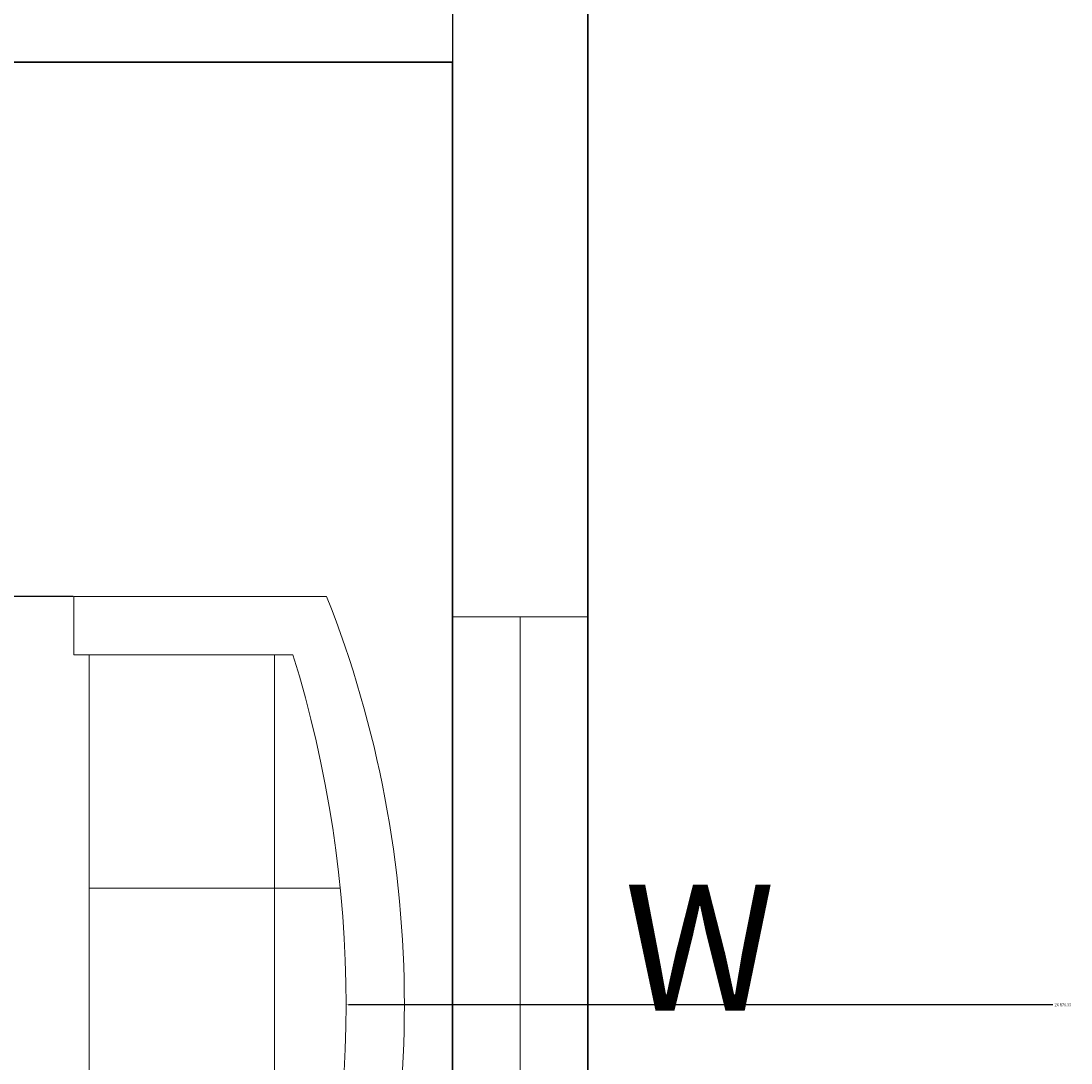
# Model space of a CAD drawing. Units: feet. Extents: x 1654 to 2985, y 1348 to 2230.
# Tile 39 of 53: x 2173 to 2243, y 1820 to 1889. Entities that reach past the tile are written whole.
import ezdxf

# ---------------------------------------------------------------- set-up
doc = ezdxf.new("R2010")
doc.units = ezdxf.units.FT
for name, color, linetype, lineweight in [('A-ANNO-DIMS', 2, 'Continuous', 18), ('A-ANNO-TEXT', 7, 'Continuous', 18), ('A-FURN', 8, 'Continuous', 13), ('A-GLAZ', 4, 'Continuous', 18), ('A-WALL', 7, 'Continuous', 35)]:
    doc.layers.add(name, color=color, linetype=linetype, lineweight=lineweight)
doc.styles.get("Standard").update_dxf_attribs({"font": 'arial.ttf'})
doc.dimstyles.get("Standard").update_dxf_attribs({"dimtxt": 0.18, "dimasz": 0.18, "dimexe": 0.18, "dimexo": 0.0625, "dimgap": 0.09, "dimtad": 0, "dimtih": 1, "dimtoh": 1, "dimdec": 4, "dimzin": 0, "dimdsep": 46, "dimtxsty": 'Standard', "dimcen": 0.09, "dimadec": 0, "dimazin": 0, "dimtfac": 1, "dimtdec": 4, "dimtofl": 0, "dimtmove": 0, "dimatfit": 3, "dimfxl": 1, "dimtolj": 1, "dimtzin": 0, "dimarcsym": 0})

# ---------------------------------------------------------------- blocks, each defined once
blk = doc.blocks.new('Sofa - Roundback 7 ft.')
for p, q in [((-12.00002, -32.4421), (-12.00003, -6.5971)), ((11.99997, -32.4421), (11.99998, -6.5971)), ((-36.000027, -34), (-36.000027, -11.4696)), ((35.99998, -34), (35.99998, -11.4696)), ((-35.999844, -13.3819), (35.9998, -13.3819)), ((-36.000027, -32.4421), (35.99998, -32.4421))]:
    blk.add_line(p, q)
for points in [[(-36.000027, -34), (-42.000027, -34), (-42.000027, -8)], [(41.99998, -8), (41.99998, -34), (35.99998, -34)]]:
    blk.add_lwpolyline(points)
for centre, radius, start, end in [((0, -114.25), 114.25, 68.43141, 111.5686), ((-0.00001, -127.1968), 121.1968, 72.72033, 107.2797)]:
    blk.add_arc(centre, radius, start, end)
blk = doc.blocks.new('WIN-LIVING-EAST')
for p, q in [((0, 47.934), (9, 47.934)), ((4.5, 47.934), (4.5, 0)), ((0, 0), (9, 0))]:
    blk.add_line(p, q)
blk = doc.blocks.new('*D38')
at = {"layer": 'A-ANNO-DIMS', "color": 0, "lineweight": -2, "transparency": 16777216}
for p, q in [((2176.839, 1850.733), (2168.575, 1850.733)), ((2168.755, 1850.553), (2168.755, 1823.764)), ((2168.755, 1796.609), (2168.755, 1823.398)), ((2176.839, 1796.429), (2168.575, 1796.429))]:
    blk.add_line(p, q, dxfattribs=at)
at = {"layer": 'A-ANNO-DIMS', "color": 0, "transparency": 16777216}
for points in [[(2168.725, 1850.553), (2168.785, 1850.553), (2168.755, 1850.733)], [(2168.725, 1796.609), (2168.785, 1796.609), (2168.755, 1796.429)]]:
    blk.add_solid(points, dxfattribs=at)
at = {"layer": 'Defpoints', "color": 0, "transparency": 16777216}
for p in [(2176.901, 1850.733), (2168.755, 1796.429), (2176.901, 1796.429)]:
    blk.add_point(p, dxfattribs=at)
at = {"layer": 'A-ANNO-DIMS', "color": 0, "transparency": 16777216, "insert": (2168.755, 1823.581), "char_height": 0.18, "attachment_point": 5}
blk.add_mtext('\\A1;SOFA 54 TYP.', dxfattribs=at)
blk = doc.blocks.new('*D80')
at = {"layer": 'A-ANNO-DIMS', "color": 0, "lineweight": -2, "transparency": 16777216}
for p, q in [((2070.092, 2039.192), (2070.092, 1534.075)), ((2202.092, 2039.192), (2202.092, 1534.075)), ((2070.272, 1534.255), (2135.813, 1534.255)), ((2201.912, 1534.255), (2136.372, 1534.255))]:
    blk.add_line(p, q, dxfattribs=at)
at = {"layer": 'A-ANNO-DIMS', "color": 0, "transparency": 16777216}
for points in [[(2070.272, 1534.285), (2070.272, 1534.225), (2070.092, 1534.255)], [(2201.912, 1534.285), (2201.912, 1534.225), (2202.092, 1534.255)]]:
    blk.add_solid(points, dxfattribs=at)
at = {"layer": 'Defpoints', "color": 0, "transparency": 16777216}
for p in [(2070.092, 2039.255), (2202.092, 2039.255), (2202.092, 1534.255)]:
    blk.add_point(p, dxfattribs=at)
at = {"layer": 'A-ANNO-DIMS', "color": 0, "transparency": 16777216, "insert": (2136.092, 1534.255), "char_height": 0.18, "attachment_point": 5}
blk.add_mtext('\\A1;132', dxfattribs=at)
blk = doc.blocks.new('*D108')
at = {"layer": 'A-ANNO-DIMS', "color": 0, "lineweight": -2, "transparency": 16777216}
for p, q in [((2116.561, 1823.581), (2116.741, 1823.581)), ((2116.651, 1823.491), (2116.651, 1823.671)), ((2242.014, 1823.581), (2195.183, 1823.581))]:
    blk.add_line(p, q, dxfattribs=at)
at = {"layer": 'A-ANNO-DIMS', "color": 0, "transparency": 16777216}
blk.add_solid([(2195.183, 1823.611), (2195.183, 1823.551), (2195.003, 1823.581)], dxfattribs=at)
at = {"layer": 'Defpoints', "color": 0, "transparency": 16777216}
for p in [(2116.651, 1823.581), (2195.003, 1823.581)]:
    blk.add_point(p, dxfattribs=at)
at = {"layer": 'A-ANNO-DIMS', "color": 0, "transparency": 16777216, "insert": (2242.689, 1823.581), "char_height": 0.18, "attachment_point": 5}
blk.add_mtext('\\A1;2X R78.35', dxfattribs=at)

msp = doc.modelspace()

# ---------------------------------------------------------------- linework, layer by layer
at = {"layer": 'A-WALL'}
for p, q in [((2211.0924, 2117.2549), (2211.0924, 1742.2549)), ((2202.0924, 1886.2549), (2070.0924, 1886.2549)), ((2202.0924, 1886.2549), (2202.0924, 1751.2549)), ((2211.0924, 1886.2549), (2211.0924, 1565.2549))]:
    msp.add_line(p, q, dxfattribs=at)

# ---------------------------------------------------------------- block references
at = {"layer": 'A-FURN', "xscale": 0.6464854603293951, "yscale": 0.6464854603293951, "zscale": 0.6464854603293951, "rotation": 270}
msp.add_blockref('Sofa - Roundback 7 ft.', (2198.8816, 1823.581), dxfattribs=at)
at = {"layer": 'A-GLAZ'}
msp.add_blockref('WIN-LIVING-EAST', (2202.092, 1801.437), dxfattribs=at)

# ---------------------------------------------------------------- texts
at = {"layer": 'A-ANNO-TEXT'}
msp.add_text('W', height=8.3811, dxfattribs=at).set_placement((2213.5177, 1823.1912))

# ---------------------------------------------------------------- dimensions: what is measured, and where the dimension line sits
at = {"layer": 'A-ANNO-DIMS'}
dim = msp.add_linear_dim(base=(2202.0924, 1534.2549), p1=(2070.0924, 2039.2549), p2=(2202.0924, 2039.2549), dimstyle='Standard', override={"dimdec": 0, "dimlfac": 1, "dimrnd": 0, "dimzin": 0, "dimdsep": 46, "dimlunit": 2}, dxfattribs=at)
dim.commit()
dim.dimension.update_dxf_attribs({"geometry": '*D80', "text_midpoint": (2136.0924, 1534.2549)})
dim = msp.add_linear_dim(base=(2168.7554, 1796.4287), p1=(2176.9011, 1850.7334), p2=(2176.9011, 1796.4287), angle=270, text='SOFA <> TYP.', dimstyle='Standard', override={"dimdec": 0, "dimlfac": 1, "dimrnd": 0, "dimzin": 0, "dimdsep": 46, "dimlunit": 2}, dxfattribs=at)
dim.commit()
dim.dimension.update_dxf_attribs({"geometry": '*D38', "text_midpoint": (2168.7554, 1823.5811)})
dim = msp.add_radius_dim(center=(2116.6507, 1823.581), mpoint=(2195.0027, 1823.581), text='2X <>', dimstyle='Standard', override={"dimdec": 2, "dimlfac": 1, "dimrnd": 0, "dimzin": 0, "dimdsep": 46, "dimlunit": 2}, dxfattribs=at)
dim.commit()
dim.dimension.update_dxf_attribs({"geometry": '*D108', "text_midpoint": (2242.0138, 1823.581), "dimtype": 164})

doc.saveas('drawing.dxf')
